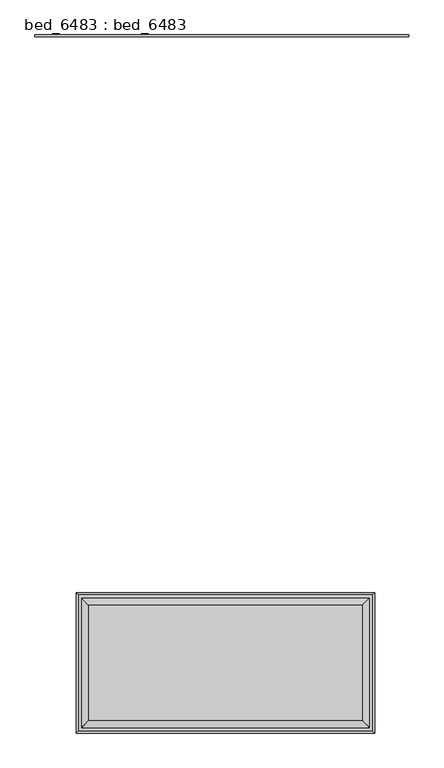
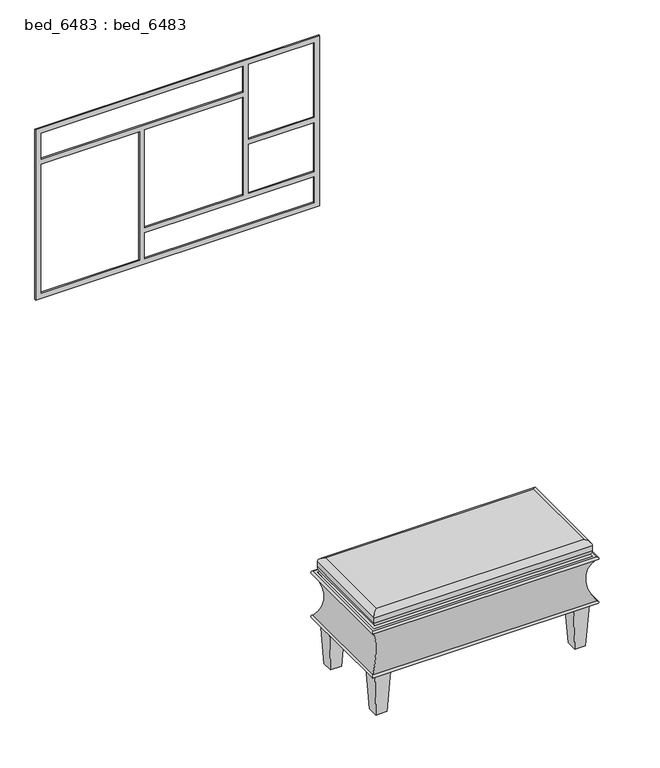
"""IFC4 building model written with IfcOpenShell, lengths in millimetres: proxy geometry, bed_6483 : bed_6483."""

from ifc_helpers import new_model, si_unit, frame, origin, place, context, project, spatial, polyline, ellipse_curve, outline, extrude, source, transform, mapped, element, save
from ifc_brep_helpers import plane_surface, cylinder_surface, revolved_surface, advanced_brep


def bed_6483_bed_6483_60f1e3ed(model_context):
    return source(origin(), model_context, "Body", "SolidModel", [
        advanced_brep(
        [(396.3268225, -944.0475635, 228.6), (396.3268225, -944.0475635, 431.8), (396.3268225, -1426.6475635, 431.8), (396.3268225, -1426.6475635, 228.6), (312.4741919, -1027.9001941, 431.8), (312.4741919, -1027.9001941, 228.6), (312.4741919, -1040.6001941, 228.6), (312.4741919, -1330.094933, 228.6), (312.4741919, -1342.794933, 228.6), (312.4741919, -1342.794933, 431.8), (-645.0731775, -1426.6475635, 431.8), (-645.0731775, -1426.6475635, 228.6), (299.7741919, -1342.794933, 228.6), (-548.520547, -1342.794933, 228.6), (-561.220547, -1342.794933, 228.6), (-561.220547, -1342.794933, 431.8), (-645.0731775, -944.0475635, 431.8), (-645.0731775, -944.0475635, 228.6), (-561.220547, -1330.094933, 228.6), (-561.220547, -1040.6001941, 228.6), (-561.220547, -1027.9001941, 228.6), (-561.220547, -1027.9001941, 431.8), (-624.720547, -1406.294933, 228.6), (-548.520547, -1406.294933, 228.6), (299.7741919, -1406.294933, 228.6), (375.9741919, -1406.294933, 228.6), (375.9741919, -1330.094933, 228.6), (375.9741919, -1040.6001941, 228.6), (375.9741919, -964.4001941, 228.6), (299.7741919, -964.4001941, 228.6), (299.7741919, -1027.9001941, 228.6), (-548.520547, -1027.9001941, 228.6), (-548.520547, -964.4001941, 228.6), (-624.720547, -964.4001941, 228.6), (-624.720547, -1040.6001941, 228.6), (-624.720547, -1330.094933, 228.6), (-632.3731775, -956.7475635, 431.8), (383.6268225, -956.7475635, 431.8), (383.6268225, -1413.9475635, 431.8), (-632.3731775, -1413.9475635, 431.8), (-548.520547, -1330.094933, 228.6), (-612.020547, -1393.594933, 0.0), (-612.020547, -1342.794933, 0.0), (-561.220547, -1342.794933, 0.0), (-561.220547, -1393.594933, 0.0), (-548.520547, -1040.6001941, 228.6), (-612.020547, -1027.9001941, 0.0), (-612.020547, -977.1001941, 0.0), (-561.220547, -977.1001941, 0.0), (-561.220547, -1027.9001941, 0.0), (299.7741919, -1330.094933, 228.6), (312.4741919, -1393.594933, 0.0), (312.4741919, -1342.794933, 0.0), (363.2741919, -1342.794933, 0.0), (363.2741919, -1393.594933, 0.0), (299.7741919, -1040.6001941, 228.6), (312.4741919, -1027.9001941, 0.0), (312.4741919, -977.1001941, 0.0), (363.2741919, -977.1001941, 0.0), (363.2741919, -1027.9001941, 0.0), (383.6268225, -956.7475635, 444.5), (-632.3731775, -956.7475635, 444.5), (-632.3731775, -1413.9475635, 444.5), (383.6268225, -1413.9475635, 444.5)],
        [
            (0, 1, ellipse_curve(frame((532.9682979, -807.4060882, 330.2), z_axis=(-0.7071067811865475, 0.7071067811865475, 0.0), x_axis=(-0.7071067811865474, -0.7071067811865476, 0.0)), 240.8047042, 170.2746393)),
            (1, 2),
            (2, 3, ellipse_curve(frame((532.9682979, -1563.2890389, 330.2), z_axis=(-0.7071067811865475, -0.7071067811865475, 0.0), x_axis=(0.7071067811865474, -0.7071067811865476, 0.0)), 240.8047042, 170.2746393)),
            (3, 0),
            (4, 5),
            (5, 6),
            (6, 7),
            (7, 8),
            (8, 9),
            (9, 4),
            (2, 10),
            (10, 11, ellipse_curve(frame((-781.7146529, -1563.2890389, 330.2), z_axis=(-0.7071067811865475, 0.7071067811865475, 0.0), x_axis=(-0.7071067811865476, -0.7071067811865474, 0.0)), 240.8047042, 170.2746393)),
            (11, 3),
            (8, 12),
            (12, 13),
            (13, 14),
            (14, 15),
            (15, 9),
            (10, 16),
            (16, 17, ellipse_curve(frame((-781.7146529, -807.4060882, 330.2), z_axis=(0.7071067811865475, 0.7071067811865475, 0.0), x_axis=(-0.7071067811865474, 0.7071067811865476, 0.0)), 240.8047042, 170.2746393)),
            (17, 11),
            (14, 18),
            (18, 19),
            (19, 20),
            (20, 21),
            (21, 15),
            (0, 17),
            (16, 1),
            (22, 23),
            (23, 13),
            (12, 24),
            (24, 25),
            (25, 26),
            (26, 7),
            (6, 27),
            (27, 28),
            (28, 29),
            (29, 30),
            (30, 31),
            (31, 32),
            (32, 33),
            (33, 34),
            (34, 19),
            (18, 35),
            (35, 22),
            (4, 21),
            (20, 31),
            (30, 5),
            (36, 37),
            (37, 38),
            (38, 39),
            (39, 36),
            (13, 40),
            (40, 18),
            (41, 42),
            (42, 43),
            (43, 44),
            (44, 41),
            (44, 23),
            (22, 41),
            (43, 40),
            (42, 35),
            (19, 45),
            (45, 31),
            (46, 47),
            (47, 48),
            (48, 49),
            (49, 46),
            (49, 45),
            (34, 46),
            (48, 32),
            (47, 33),
            (7, 50),
            (50, 12),
            (51, 52),
            (52, 53),
            (53, 54),
            (54, 51),
            (54, 25),
            (24, 51),
            (53, 26),
            (52, 50),
            (55, 6),
            (30, 55),
            (56, 57),
            (57, 58),
            (58, 59),
            (59, 56),
            (59, 27),
            (55, 56),
            (58, 28),
            (57, 29),
            (60, 61),
            (61, 62),
            (62, 63),
            (63, 60),
            (60, 37),
            (36, 61),
            (39, 62),
            (38, 63),
        ],
        [
            revolved_surface(polyline([(703.2429372, -1733.5636781814405, 330.2), (703.2429372, -637.1314489185593, 330.2)]), (532.9682979, -944.0475635, 330.2), (0.0, -1.0, 0.0)),
            plane_surface(frame((312.4741919, -1027.9001941, 228.6), z_axis=(-1.0, 0.0, 0.0), x_axis=(0.0, -1.0, 0.0))),
            revolved_surface(polyline([(-951.989292181441, -1733.5636782, 330.2), (703.2429371814408, -1733.5636782, 330.2)]), (396.3268225, -1563.2890389, 330.2), (-1.0, 0.0, 0.0)),
            plane_surface(frame((312.4741919, -1342.794933, 228.6), z_axis=(0.0, 1.0, 0.0), x_axis=(-1.0, 0.0, 0.0))),
            revolved_surface(polyline([(-951.9892922, -637.1314489185593, 330.2), (-951.9892922, -1733.5636781814405, 330.2)]), (-781.7146529, -1426.6475635, 330.2), (0.0, 1.0, 0.0)),
            plane_surface(frame((-561.220547, -1342.794933, 228.6), z_axis=(1.0, 0.0, 0.0), x_axis=(0.0, 1.0, 0.0))),
            revolved_surface(polyline([(703.2429371814407, -637.1314489, 330.2), (-951.9892921814408, -637.1314489, 330.2)]), (-645.0731775, -807.4060882, 330.2), (1.0, 0.0, 0.0)),
            plane_surface(frame((-645.0731775, -944.0475635, 228.6), z_axis=(0.0, 0.0, -1.0), x_axis=(1.0, 0.0, 0.0))),
            plane_surface(frame((-561.220547, -1027.9001941, 228.6), z_axis=(0.0, -1.0, 0.0), x_axis=(1.0, 0.0, 0.0))),
            plane_surface(frame((-561.220547, -1027.9001941, 431.8), z_axis=(0.0, 0.0, 1.0), x_axis=(1.0, 0.0, 0.0))),
            plane_surface(frame((-586.620547, -1368.194933, 228.6), z_axis=(0.0, 0.0, 1.0), x_axis=(1.0, 0.0, 0.0))),
            plane_surface(frame((-586.620547, -1368.194933, 0.0), z_axis=(0.0, 0.0, -1.0), x_axis=(1.0, 0.0, 0.0))),
            plane_surface(frame((-586.620547, -1393.594933, 0.0), z_axis=(0.0, -0.9984603532054125, -0.055470019622523306), x_axis=(1.0, 0.0, 0.0))),
            plane_surface(frame((-561.220547, -1368.194933, 0.0), z_axis=(0.9984603532054125, 0.0, -0.05547001962252301), x_axis=(0.0, 1.0, 0.0))),
            plane_surface(frame((-586.620547, -1342.794933, 0.0), z_axis=(0.0, 0.9984603532054125, -0.05547001962252228), x_axis=(-1.0, 0.0, 0.0))),
            plane_surface(frame((-612.020547, -1368.194933, 0.0), z_axis=(-0.9984603532054125, 0.0, -0.0554700196225223), x_axis=(0.0, -1.0, 0.0))),
            plane_surface(frame((-586.620547, -1002.5001941, 228.6), z_axis=(0.0, 0.0, 1.0), x_axis=(1.0, 0.0, 0.0))),
            plane_surface(frame((-586.620547, -1002.5001941, 0.0), z_axis=(0.0, 0.0, -1.0), x_axis=(1.0, 0.0, 0.0))),
            plane_surface(frame((-586.620547, -1027.9001941, 0.0), z_axis=(0.0, -0.9984603532054125, -0.055470019622523306), x_axis=(1.0, 0.0, 0.0))),
            plane_surface(frame((-561.220547, -1002.5001941, 0.0), z_axis=(0.9984603532054125, 0.0, -0.05547001962252301), x_axis=(0.0, 1.0, 0.0))),
            plane_surface(frame((-586.620547, -977.1001941, 0.0), z_axis=(0.0, 0.9984603532054125, -0.05547001962252228), x_axis=(-1.0, 0.0, 0.0))),
            plane_surface(frame((-612.020547, -1002.5001941, 0.0), z_axis=(-0.9984603532054125, 0.0, -0.05547001962252171), x_axis=(0.0, -1.0, 0.0))),
            plane_surface(frame((337.8741919, -1368.194933, 228.6), z_axis=(0.0, 0.0, 1.0), x_axis=(1.0, 0.0, 0.0))),
            plane_surface(frame((337.8741919, -1368.194933, 0.0), z_axis=(0.0, 0.0, -1.0), x_axis=(1.0, 0.0, 0.0))),
            plane_surface(frame((337.8741919, -1393.594933, 0.0), z_axis=(0.0, -0.9984603532054125, -0.055470019622523306), x_axis=(1.0, 0.0, 0.0))),
            plane_surface(frame((363.2741919, -1368.194933, 0.0), z_axis=(0.9984603532054125, 0.0, -0.05547001962252301), x_axis=(0.0, 1.0, 0.0))),
            plane_surface(frame((337.8741919, -1342.794933, 0.0), z_axis=(0.0, 0.9984603532054125, -0.05547001962252228), x_axis=(-1.0, 0.0, 0.0))),
            plane_surface(frame((312.4741919, -1368.194933, 0.0), z_axis=(-0.9984603532054125, 0.0, -0.0554700196225223), x_axis=(0.0, -1.0, 0.0))),
            plane_surface(frame((337.8741919, -1002.5001941, 228.6), z_axis=(0.0, 0.0, 1.0), x_axis=(1.0, 0.0, 0.0))),
            plane_surface(frame((337.8741919, -1002.5001941, 0.0), z_axis=(0.0, 0.0, -1.0), x_axis=(1.0, 0.0, 0.0))),
            plane_surface(frame((337.8741919, -1027.9001941, 0.0), z_axis=(0.0, -0.9984603532054125, -0.055470019622523306), x_axis=(1.0, 0.0, 0.0))),
            plane_surface(frame((363.2741919, -1002.5001941, 0.0), z_axis=(0.9984603532054125, 0.0, -0.05547001962252301), x_axis=(0.0, 1.0, 0.0))),
            plane_surface(frame((337.8741919, -977.1001941, 0.0), z_axis=(0.0, 0.9984603532054125, -0.05547001962252228), x_axis=(-1.0, 0.0, 0.0))),
            plane_surface(frame((312.4741919, -1002.5001941, 0.0), z_axis=(-0.9984603532054125, 0.0, -0.0554700196225223), x_axis=(0.0, -1.0, 0.0))),
            plane_surface(frame((-632.3731775, -956.7475635, 444.5), z_axis=(0.0, 0.0, 1.0), x_axis=(-1.0, 0.0, 0.0))),
            plane_surface(frame((-632.3731775, -956.7475635, 431.8), z_axis=(0.0, 0.0, -1.0), x_axis=(1.0, 0.0, 0.0))),
            plane_surface(frame((383.6268225, -956.7475635, 444.5), z_axis=(0.0, 1.0, 0.0), x_axis=(0.0, 0.0, -1.0))),
            plane_surface(frame((-632.3731775, -956.7475635, 444.5), z_axis=(-1.0, 0.0, 0.0), x_axis=(0.0, 0.0, -1.0))),
            plane_surface(frame((-632.3731775, -1413.9475635, 444.5), z_axis=(0.0, -1.0, 0.0), x_axis=(0.0, 0.0, -1.0))),
            plane_surface(frame((383.6268225, -1413.9475635, 444.5), z_axis=(1.0, 0.0, 0.0), x_axis=(0.0, 0.0, -1.0))),
        ],
        [
            (0, [[1, 2, 3, 4]]),
            (1, [[5, 6, 7, 8, 9, 10]]),
            (2, [[-3, 11, 12, 13]]),
            (3, [[-9, 14, 15, 16, 17, 18]]),
            (4, [[-12, 19, 20, 21]]),
            (5, [[-17, 22, 23, 24, 25, 26]]),
            (6, [[-1, 27, -20, 28]]),
            (7, [[-4, -13, -21, -27], [29, 30, -15, 31, 32, 33, 34, -7, 35, 36, 37, 38, 39, 40, 41, 42, 43, -23, 44, 45]]),
            (8, [[-5, 46, -25, 47, -39, 48]]),
            (9, [[-2, -28, -19, -11], [49, 50, 51, 52]]),
            (10, [[53, 54, -22, -16]]),
            (11, [[55, 56, 57, 58]]),
            (12, [[-58, 59, -29, 60]]),
            (13, [[-57, 61, -53, -30, -59]]),
            (14, [[-56, 62, -44, -54, -61]]),
            (15, [[-55, -60, -45, -62]]),
            (16, [[63, 64, -47, -24]]),
            (17, [[65, 66, 67, 68]]),
            (18, [[-68, 69, -63, -43, 70]]),
            (19, [[-67, 71, -40, -64, -69]]),
            (20, [[-66, 72, -41, -71]]),
            (21, [[-65, -70, -42, -72]]),
            (22, [[73, 74, -14, -8]]),
            (23, [[75, 76, 77, 78]]),
            (24, [[-78, 79, -32, 80]]),
            (25, [[-77, 81, -33, -79]]),
            (26, [[-76, 82, -73, -34, -81]]),
            (27, [[-75, -80, -31, -74, -82]]),
            (28, [[83, -6, -48, 84]]),
            (29, [[85, 86, 87, 88]]),
            (30, [[-88, 89, -35, -83, 90]]),
            (31, [[-87, 91, -36, -89]]),
            (32, [[-86, 92, -37, -91]]),
            (33, [[-85, -90, -84, -38, -92]]),
            (34, [[93, 94, 95, 96]]),
            (35, [[-10, -18, -26, -46]]),
            (36, [[-93, 97, -49, 98]]),
            (37, [[-94, -98, -52, 99]]),
            (38, [[-95, -99, -51, 100]]),
            (39, [[-96, -100, -50, -97]]),
        ],
    ),
        advanced_brep(
        [(383.6268225, -956.7475635, 228.6), (383.6268225, -956.7475635, 215.9), (383.6268225, -1413.9475635, 215.9), (383.6268225, -1413.9475635, 228.6), (396.3268225, -944.0475635, 215.9), (396.3268225, -944.0475635, 228.6), (396.3268225, -1426.6475635, 228.6), (396.3268225, -1426.6475635, 215.9), (-632.3731775, -1413.9475635, 215.9), (-632.3731775, -1413.9475635, 228.6), (-645.0731775, -1426.6475635, 228.6), (-645.0731775, -1426.6475635, 215.9), (-632.3731775, -956.7475635, 215.9), (-632.3731775, -956.7475635, 228.6), (-645.0731775, -944.0475635, 228.6), (-645.0731775, -944.0475635, 215.9)],
        [
            (0, 1),
            (1, 2),
            (2, 3),
            (3, 0),
            (4, 5, ellipse_curve(frame((396.3268225, -944.0475635, 222.25), z_axis=(0.7071067811865476, -0.7071067811865474, 0.0), x_axis=(0.7071067811865474, 0.7071067811865478, 0.0)), 8.9802561, 6.35)),
            (5, 6),
            (6, 7, ellipse_curve(frame((396.3268225, -1426.6475635, 222.25), z_axis=(0.7071067811865475, 0.7071067811865476, 0.0), x_axis=(-0.7071067811865475, 0.7071067811865475, 0.0)), 8.9802561, 6.35)),
            (7, 4),
            (2, 8),
            (8, 9),
            (9, 3),
            (6, 10),
            (10, 11, ellipse_curve(frame((-645.0731775, -1426.6475635, 222.25), z_axis=(0.7071067811865476, -0.7071067811865475, 0.0), x_axis=(0.7071067811865475, 0.7071067811865475, 0.0)), 8.9802561, 6.35)),
            (11, 7),
            (8, 12),
            (12, 13),
            (13, 9),
            (10, 14),
            (14, 15, ellipse_curve(frame((-645.0731775, -944.0475635, 222.25), z_axis=(-0.7071067811865474, -0.7071067811865476, 0.0), x_axis=(0.7071067811865475, -0.7071067811865476, 0.0)), 8.9802561, 6.35)),
            (15, 11),
            (15, 4),
            (1, 12),
            (0, 13),
            (5, 14),
        ],
        [
            plane_surface(frame((383.6268225, -956.7475635, 215.9), z_axis=(-1.0, 0.0, 0.0), x_axis=(0.0, -1.0, 0.0))),
            cylinder_surface(frame((396.3268225, -944.0475635, 222.25), z_axis=(0.0, 1.0, 0.0), x_axis=(-1.0, 0.0, 0.0)), 6.35),
            plane_surface(frame((383.6268225, -1413.9475635, 215.9), z_axis=(0.0, 1.0, 0.0), x_axis=(-1.0, 0.0, 0.0))),
            cylinder_surface(frame((396.3268225, -1426.6475635, 222.25), z_axis=(1.0, 0.0, 0.0), x_axis=(0.0, 1.0, 0.0)), 6.35),
            plane_surface(frame((-632.3731775, -1413.9475635, 215.9), z_axis=(1.0, 0.0, 0.0), x_axis=(0.0, 1.0, 0.0))),
            cylinder_surface(frame((-645.0731775, -1426.6475635, 222.25), z_axis=(0.0, -1.0, 0.0), x_axis=(1.0, 0.0, 0.0)), 6.35),
            plane_surface(frame((-645.0731775, -944.0475635, 215.9), z_axis=(0.0, 0.0, -1.0), x_axis=(1.0, 0.0, 0.0))),
            plane_surface(frame((-632.3731775, -956.7475635, 215.9), z_axis=(0.0, -1.0, 0.0), x_axis=(1.0, 0.0, 0.0))),
            plane_surface(frame((-632.3731775, -956.7475635, 228.6), z_axis=(0.0, 0.0, 1.0), x_axis=(1.0, 0.0, 0.0))),
            cylinder_surface(frame((-645.0731775, -944.0475635, 222.25), z_axis=(-1.0, 0.0, 0.0), x_axis=(0.0, -1.0, 0.0)), 6.35),
        ],
        [
            (0, [[1, 2, 3, 4]]),
            (1, [[5, 6, 7, 8]]),
            (2, [[-3, 9, 10, 11]]),
            (3, [[-7, 12, 13, 14]]),
            (4, [[-10, 15, 16, 17]]),
            (5, [[-13, 18, 19, 20]]),
            (6, [[-8, -14, -20, 21], [-2, 22, -15, -9]]),
            (7, [[-1, 23, -16, -22]]),
            (8, [[-6, 24, -18, -12], [-4, -11, -17, -23]]),
            (9, [[-5, -21, -19, -24]]),
        ],
    ),
        advanced_brep(
        [(383.6268225, -956.7475635, 444.5), (383.6268225, -956.7475635, 431.8), (383.6268225, -1413.9475635, 431.8), (383.6268225, -1413.9475635, 444.5), (396.3268225, -944.0475635, 431.8), (396.3268225, -944.0475635, 444.5), (396.3268225, -1426.6475635, 444.5), (396.3268225, -1426.6475635, 431.8), (-632.3731775, -1413.9475635, 431.8), (-632.3731775, -1413.9475635, 444.5), (-645.0731775, -1426.6475635, 444.5), (-645.0731775, -1426.6475635, 431.8), (-632.3731775, -956.7475635, 431.8), (-632.3731775, -956.7475635, 444.5), (-645.0731775, -944.0475635, 444.5), (-645.0731775, -944.0475635, 431.8)],
        [
            (0, 1),
            (1, 2),
            (2, 3),
            (3, 0),
            (4, 5, ellipse_curve(frame((396.3268225, -944.0475635, 438.15), z_axis=(0.7071067811865476, -0.7071067811865474, 0.0), x_axis=(0.7071067811865474, 0.7071067811865478, 0.0)), 8.9802561, 6.35)),
            (5, 6),
            (6, 7, ellipse_curve(frame((396.3268225, -1426.6475635, 438.15), z_axis=(0.7071067811865475, 0.7071067811865476, 0.0), x_axis=(-0.7071067811865475, 0.7071067811865475, 0.0)), 8.9802561, 6.35)),
            (7, 4),
            (2, 8),
            (8, 9),
            (9, 3),
            (6, 10),
            (10, 11, ellipse_curve(frame((-645.0731775, -1426.6475635, 438.15), z_axis=(0.7071067811865476, -0.7071067811865475, 0.0), x_axis=(0.7071067811865475, 0.7071067811865475, 0.0)), 8.9802561, 6.35)),
            (11, 7),
            (8, 12),
            (12, 13),
            (13, 9),
            (10, 14),
            (14, 15, ellipse_curve(frame((-645.0731775, -944.0475635, 438.15), z_axis=(-0.7071067811865474, -0.7071067811865476, 0.0), x_axis=(0.7071067811865475, -0.7071067811865476, 0.0)), 8.9802561, 6.35)),
            (15, 11),
            (15, 4),
            (1, 12),
            (0, 13),
            (5, 14),
        ],
        [
            plane_surface(frame((383.6268225, -956.7475635, 431.8), z_axis=(-1.0, 0.0, 0.0), x_axis=(0.0, -1.0, 0.0))),
            cylinder_surface(frame((396.3268225, -944.0475635, 438.15), z_axis=(0.0, 1.0, 0.0), x_axis=(-1.0, 0.0, 0.0)), 6.35),
            plane_surface(frame((383.6268225, -1413.9475635, 431.8), z_axis=(0.0, 1.0, 0.0), x_axis=(-1.0, 0.0, 0.0))),
            cylinder_surface(frame((396.3268225, -1426.6475635, 438.15), z_axis=(1.0, 0.0, 0.0), x_axis=(0.0, 1.0, 0.0)), 6.35),
            plane_surface(frame((-632.3731775, -1413.9475635, 431.8), z_axis=(1.0, 0.0, 0.0), x_axis=(0.0, 1.0, 0.0))),
            cylinder_surface(frame((-645.0731775, -1426.6475635, 438.15), z_axis=(0.0, -1.0, 0.0), x_axis=(1.0, 0.0, 0.0)), 6.35),
            plane_surface(frame((-645.0731775, -944.0475635, 431.8), z_axis=(0.0, 0.0, -1.0), x_axis=(1.0, 0.0, 0.0))),
            plane_surface(frame((-632.3731775, -956.7475635, 431.8), z_axis=(0.0, -1.0, 0.0), x_axis=(1.0, 0.0, 0.0))),
            plane_surface(frame((-632.3731775, -956.7475635, 444.5), z_axis=(0.0, 0.0, 1.0), x_axis=(1.0, 0.0, 0.0))),
            cylinder_surface(frame((-645.0731775, -944.0475635, 438.15), z_axis=(-1.0, 0.0, 0.0), x_axis=(0.0, -1.0, 0.0)), 6.35),
        ],
        [
            (0, [[1, 2, 3, 4]]),
            (1, [[5, 6, 7, 8]]),
            (2, [[-3, 9, 10, 11]]),
            (3, [[-7, 12, 13, 14]]),
            (4, [[-10, 15, 16, 17]]),
            (5, [[-13, 18, 19, 20]]),
            (6, [[-8, -14, -20, 21], [-2, 22, -15, -9]]),
            (7, [[-1, 23, -16, -22]]),
            (8, [[-6, 24, -18, -12], [-4, -11, -17, -23]]),
            (9, [[-5, -21, -19, -24]]),
        ],
    ),
        advanced_brep(
        [(-606.9731775, -1388.5475635, 520.7), (358.2268225, -1388.5475635, 520.7), (358.2268225, -982.1475635, 520.7), (-606.9731775, -982.1475635, 520.7), (358.2268225, -1388.5475635, 444.5), (-606.9731775, -1388.5475635, 444.5), (-606.9731775, -982.1475635, 444.5), (358.2268225, -982.1475635, 444.5), (383.6268225, -956.7475635, 495.3), (383.6268225, -956.7475635, 469.9), (-632.3731775, -956.7475635, 469.9), (-632.3731775, -956.7475635, 495.3), (-632.3731775, -1413.9475635, 469.9), (-632.3731775, -1413.9475635, 495.3), (383.6268225, -1413.9475635, 469.9), (383.6268225, -1413.9475635, 495.3)],
        [
            (0, 1),
            (1, 2),
            (2, 3),
            (3, 0),
            (4, 5),
            (5, 6),
            (6, 7),
            (7, 4),
            (8, 9),
            (9, 10),
            (10, 11),
            (11, 8),
            (10, 12),
            (12, 13),
            (13, 11),
            (12, 14),
            (14, 15),
            (15, 13),
            (8, 15),
            (14, 9),
            (15, 1, ellipse_curve(frame((358.2268225, -1388.5475635, 495.3), z_axis=(-0.7071067811865475, -0.7071067811865475, 0.0), x_axis=(0.7071067811865476, -0.7071067811865474, 0.0)), 35.9210245, 25.4)),
            (0, 13, ellipse_curve(frame((-606.9731775, -1388.5475635, 495.3), z_axis=(0.7071067811865475, -0.7071067811865475, 0.0), x_axis=(0.7071067811865476, 0.7071067811865474, 0.0)), 35.9210245, 25.4)),
            (4, 14, ellipse_curve(frame((358.2268225, -1388.5475635, 469.9), z_axis=(-0.7071067811865475, -0.7071067811865475, 0.0), x_axis=(0.7071067811865476, -0.7071067811865474, 0.0)), 35.9210245, 25.4)),
            (12, 5, ellipse_curve(frame((-606.9731775, -1388.5475635, 469.9), z_axis=(0.7071067811865475, -0.7071067811865475, 0.0), x_axis=(0.7071067811865476, 0.7071067811865474, 0.0)), 35.9210245, 25.4)),
            (8, 2, ellipse_curve(frame((358.2268225, -982.1475635, 495.3), z_axis=(0.7071067811865475, -0.7071067811865475, 0.0), x_axis=(0.7071067811865474, 0.7071067811865476, 0.0)), 35.9210245, 25.4)),
            (7, 9, ellipse_curve(frame((358.2268225, -982.1475635, 469.9), z_axis=(0.7071067811865475, -0.7071067811865475, 0.0), x_axis=(0.7071067811865474, 0.7071067811865476, 0.0)), 35.9210245, 25.4)),
            (11, 3, ellipse_curve(frame((-606.9731775, -982.1475635, 495.3), z_axis=(0.7071067811865475, 0.7071067811865475, 0.0), x_axis=(-0.7071067811865476, 0.7071067811865474, 0.0)), 35.9210245, 25.4)),
            (6, 10, ellipse_curve(frame((-606.9731775, -982.1475635, 469.9), z_axis=(0.7071067811865475, 0.7071067811865475, 0.0), x_axis=(-0.7071067811865476, 0.7071067811865474, 0.0)), 35.9210245, 25.4)),
        ],
        [
            plane_surface(frame((-632.3731775, -956.7475635, 520.7), z_axis=(0.0, 0.0, 1.0), x_axis=(-1.0, 0.0, 0.0))),
            plane_surface(frame((-632.3731775, -956.7475635, 444.5), z_axis=(0.0, 0.0, -1.0), x_axis=(1.0, 0.0, 0.0))),
            plane_surface(frame((383.6268225, -956.7475635, 520.7), z_axis=(0.0, 1.0, 0.0), x_axis=(0.0, 0.0, -1.0))),
            plane_surface(frame((-632.3731775, -956.7475635, 520.7), z_axis=(-1.0, 0.0, 0.0), x_axis=(0.0, 0.0, -1.0))),
            plane_surface(frame((-632.3731775, -1413.9475635, 520.7), z_axis=(0.0, -1.0, 0.0), x_axis=(0.0, 0.0, -1.0))),
            plane_surface(frame((383.6268225, -1413.9475635, 520.7), z_axis=(1.0, 0.0, 0.0), x_axis=(0.0, 0.0, -1.0))),
            cylinder_surface(frame((-632.3731775, -1388.5475635, 495.3), z_axis=(1.0, 0.0, 0.0), x_axis=(0.0, 1.0, 0.0)), 25.4),
            cylinder_surface(frame((-632.3731775, -1388.5475635, 469.9), z_axis=(1.0, 0.0, 0.0), x_axis=(0.0, 1.0, 0.0)), 25.4),
            cylinder_surface(frame((358.2268225, -1413.9475635, 495.3), z_axis=(0.0, 1.0, 0.0), x_axis=(-1.0, 0.0, 0.0)), 25.4),
            cylinder_surface(frame((358.2268225, -1413.9475635, 469.9), z_axis=(0.0, 1.0, 0.0), x_axis=(-1.0, 0.0, 0.0)), 25.4),
            cylinder_surface(frame((383.6268225, -982.1475635, 495.3), z_axis=(-1.0, 0.0, 0.0), x_axis=(0.0, -1.0, 0.0)), 25.4),
            cylinder_surface(frame((383.6268225, -982.1475635, 469.9), z_axis=(-1.0, 0.0, 0.0), x_axis=(0.0, -1.0, 0.0)), 25.4),
            cylinder_surface(frame((-606.9731775, -956.7475635, 495.3), z_axis=(0.0, -1.0, 0.0), x_axis=(1.0, 0.0, 0.0)), 25.4),
            cylinder_surface(frame((-606.9731775, -956.7475635, 469.9), z_axis=(0.0, -1.0, 0.0), x_axis=(1.0, 0.0, 0.0)), 25.4),
        ],
        [
            (0, [[1, 2, 3, 4]]),
            (1, [[5, 6, 7, 8]]),
            (2, [[9, 10, 11, 12]]),
            (3, [[-11, 13, 14, 15]]),
            (4, [[-14, 16, 17, 18]]),
            (5, [[-9, 19, -17, 20]]),
            (6, [[21, -1, 22, -18]]),
            (7, [[23, -16, 24, -5]]),
            (8, [[-21, -19, 25, -2]]),
            (9, [[-23, -8, 26, -20]]),
            (10, [[-25, -12, 27, -3]]),
            (11, [[-26, -7, 28, -10]]),
            (12, [[-22, -4, -27, -15]]),
            (13, [[-24, -13, -28, -6]]),
        ],
    ),
        extrude(outline(polyline([(636.5875, -797.3359102), (636.5875, 523.4640898), (1473.2, 523.4640898), (1473.2, -797.3359102), (636.5875, -797.3359102)]), holes=[polyline([(661.9875, -771.9359102), (1295.4, -771.9359102), (1295.4, -314.7359102), (661.9875, -314.7359102), (661.9875, -771.9359102)]), polyline([(1447.8, 167.8640898), (1320.8, 167.8640898), (1320.8, -771.9359102), (1447.8, -771.9359102), (1447.8, 167.8640898)]), polyline([(1295.4, 167.8640898), (814.3875, 167.8640898), (814.3875, -289.3359102), (1295.4, -289.3359102), (1295.4, 167.8640898)]), polyline([(788.9875, 498.0640898), (661.9875, 498.0640898), (661.9875, -289.3359102), (788.9875, -289.3359102), (788.9875, 498.0640898)]), polyline([(814.3875, 193.2640898), (1054.89375, 193.2640898), (1054.89375, 498.0640898), (814.3875, 498.0640898), (814.3875, 193.2640898)]), polyline([(1447.8, 498.0640898), (1080.29375, 498.0640898), (1080.29375, 193.2640898), (1447.8, 193.2640898), (1447.8, 498.0640898)])]), frame((0.0, 1026.3248059, 0.0), z_axis=(0.0, 1.0, 0.0), x_axis=(0.0, 0.0, 1.0)), (0.0, 0.0, 1.0), 6.35),
    ])


if __name__ == "__main__":
    model = new_model("IFC4")
    model_context = context("Model", 3, world=origin())
    ifc_project = project(units=[si_unit("LENGTHUNIT", "METRE", prefix="MILLI")], contexts=[model_context])
    site = spatial("IfcSite", under=ifc_project)
    building = spatial("IfcBuilding", under=site)
    placement = place(None, origin())
    bed_6483_bed_6483_shape = bed_6483_bed_6483_60f1e3ed(model_context)
    element("IfcBuildingElementProxy", 1, Name="bed_6483 : bed_6483", ObjectType="bed_6483 : bed_6483", at=placement, inside=building, context=model_context, shape_type="MappedRepresentation", body=[
        mapped(bed_6483_bed_6483_shape, transform((0.0, 0.0, 0.0), x_axis=(1.0, 0.0, 0.0), y_axis=(0.0, 1.0, 0.0), z_axis=(0.0, 0.0, 1.0))),
    ])
    save(model, "model.ifc")

# Revit data of these elements
# Type "bed_6483 : bed_6483"
#   wood = none
#   fabric 2 [instance default] = none
#   fabric [instance default] = none
#   Mirror = none
#   Default Elevation = 0
# Element 1 (IfcBuildingElementProxy, "bed_6483 : bed_6483")
#   Materials on its faces: "wood", "fabric", "fabric 2", "mirror", "chrome"
# Materials
#   "wood": class "Wood", colour RGB 71 38 7, transparency 0
#   "fabric": class "Fabric", colour RGB 56 56 56, transparency 0
#   "fabric 2": class "Fabric", colour RGB 64 0 0, transparency 0
#   "mirror": class "Glass", colour RGB 228 228 228, transparency 0.06
#   "chrome": class "Metal", colour RGB 244 244 244, transparency 0
